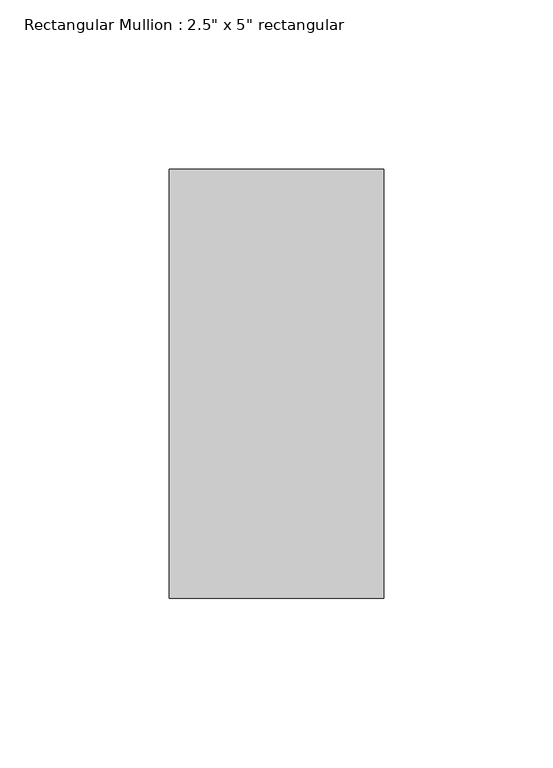
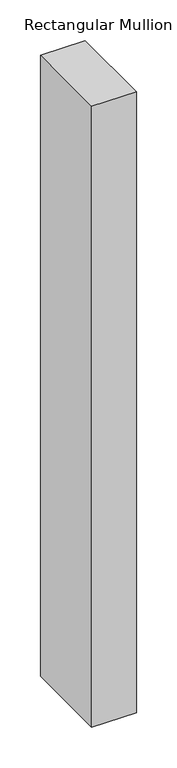
"""IFC4 building model written with IfcOpenShell, lengths in millimetres: member geometry."""

from ifc_helpers import new_model, si_unit, frame, origin, place, context, project, spatial, polyline, outline, extrude, source, transform, mapped, element, save


def member_2dd2b658(model_context):
    return source(origin(), model_context, "Body", "SweptSolid", [
        extrude(outline(polyline([(0.0, 63.5), (0.0, -63.5), (-63.5, -63.5), (-63.5, 63.5), (0.0, 63.5)])), frame((0.0, 0.0, -935.4716084), z_axis=(0.0, 0.0, 1.0), x_axis=(1.0, 0.0, 0.0)), (0.0, 0.0, 1.0), 935.4716084),
    ])


if __name__ == "__main__":
    model = new_model("IFC4")
    model_context = context("Model", 3, world=origin())
    ifc_project = project(units=[si_unit("LENGTHUNIT", "METRE", prefix="MILLI")], contexts=[model_context])
    site = spatial("IfcSite", under=ifc_project)
    building = spatial("IfcBuilding", under=site)
    placement = place(None, origin())
    member_shape = member_2dd2b658(model_context)
    element("IfcMember", 1, ObjectType="Rectangular Mullion : 2.5\" x 5\" rectangular", at=placement, inside=building, context=model_context, shape_type="MappedRepresentation", body=[
        mapped(member_shape, transform((0.0, 0.0, 0.0), x_axis=(1.0, 0.0, 0.0), y_axis=(0.0, 1.0, 0.0), z_axis=(0.0, 0.0, 1.0))),
    ])
    save(model, "model.ifc")

# Revit data of these elements
# Type "Rectangular Mullion : 2.5\" x 5\" rectangular"
#   built-in parameter 1007304 = 0.416667 (stored number, unit not read)
#   built-in parameter 1007301 = 0.104167 (stored number, unit not read)
#   built-in parameter 1007300 = 0.104167 (stored number, unit not read)
# Element 1 (IfcMember, "Rectangular Mullion : 2.5\" x 5\" rectangular")
#   Materials on its faces: "Aluminum"
# Materials
#   "Aluminum": class "Metal", colour RGB 247 247 247, transparency 0, Description = "Aluminum 6061", Cost = 0
